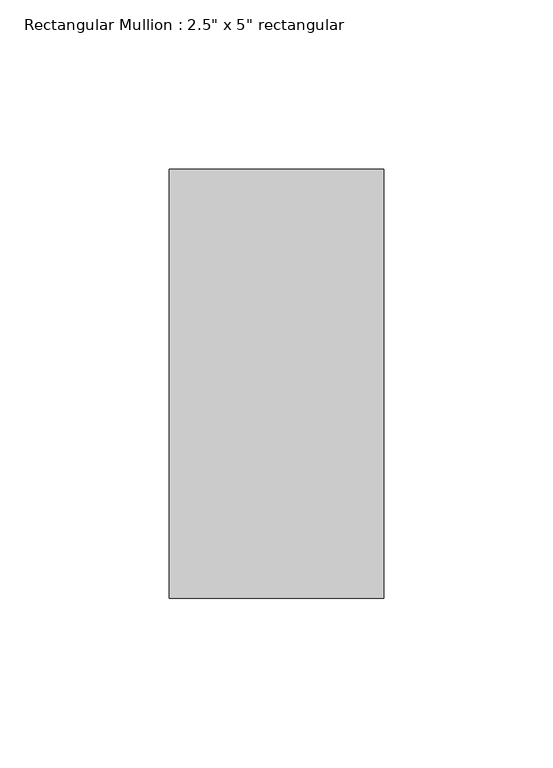
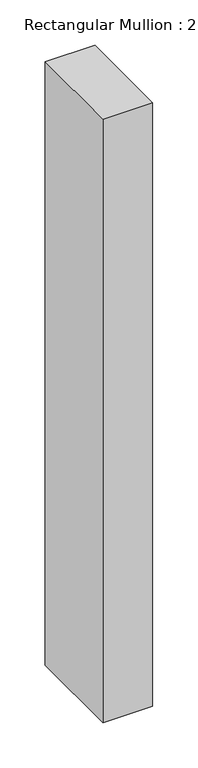
"""IFC4 building model written with IfcOpenShell, lengths in millimetres: member geometry."""

from ifc_helpers import new_model, si_unit, frame, origin, place, context, project, spatial, polyline, outline, extrude, source, transform, mapped, element, save


def member_166502d3(model_context):
    return source(origin(), model_context, "Body", "SweptSolid", [
        extrude(outline(polyline([(31.75, 63.5), (31.75, -63.5), (-31.75, -63.5), (-31.75, 63.5), (31.75, 63.5)])), frame((0.0, 0.0, -811.4673296), z_axis=(0.0, 0.0, 1.0), x_axis=(1.0, 0.0, 0.0)), (0.0, 0.0, 1.0), 811.4673296),
    ])


if __name__ == "__main__":
    model = new_model("IFC4")
    model_context = context("Model", 3, world=origin())
    ifc_project = project(units=[si_unit("LENGTHUNIT", "METRE", prefix="MILLI")], contexts=[model_context])
    site = spatial("IfcSite", under=ifc_project)
    building = spatial("IfcBuilding", under=site)
    placement = place(None, origin())
    member_shape = member_166502d3(model_context)
    element("IfcMember", 1, ObjectType="Rectangular Mullion : 2.5\" x 5\" rectangular", at=placement, inside=building, context=model_context, shape_type="MappedRepresentation", body=[
        mapped(member_shape, transform((0.0, 0.0, 0.0), x_axis=(1.0, 0.0, 0.0), y_axis=(0.0, 1.0, 0.0), z_axis=(0.0, 0.0, 1.0))),
    ])
    save(model, "model.ifc")

# Revit data of these elements
# Type "Rectangular Mullion : 2.5\" x 5\" rectangular"
#   built-in parameter 1007304 = 0.416667 (stored number, unit not read)
#   built-in parameter 1007301 = 0.104167 (stored number, unit not read)
#   built-in parameter 1007300 = 0.104167 (stored number, unit not read)
# Element 1 (IfcMember, "Rectangular Mullion : 2.5\" x 5\" rectangular")
#   Materials on its faces: "Aluminum"
# Materials
#   "Aluminum": class "Metal", colour RGB 247 247 247, transparency 0, Description = "Aluminum 6061", Cost = 0
